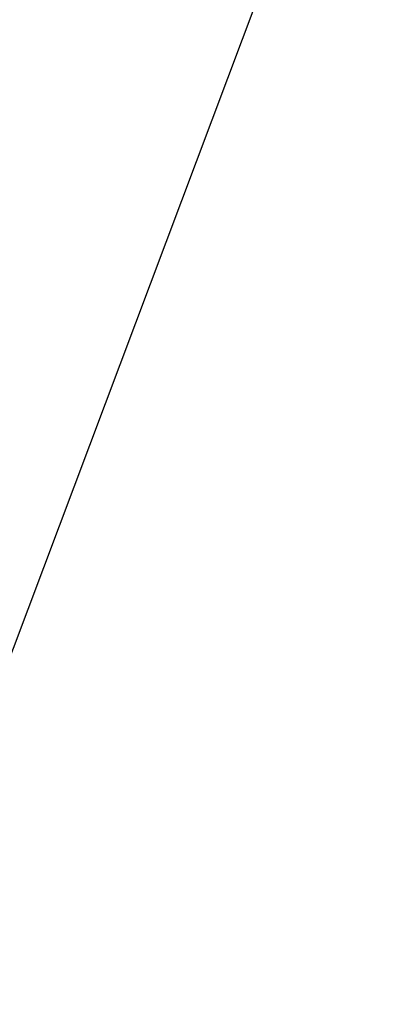
# Model space of a CAD drawing. Units: inches. Extents: x 3590 to 5167, y 65 to 1917.
# Tile 86 of 100: x 5051.6658 to 5051.8188, y 1788.6144 to 1789.0318. Entities that reach past the tile are written whole.
import ezdxf

# ---------------------------------------------------------------- set-up
doc = ezdxf.new("R2010")
doc.units = ezdxf.units.IN
for name, color, linetype, lineweight in [('A-ANNO-DIMS', 2, 'Continuous', 18), ('A-FLOR-PATT', 8, 'Continuous', 13), ('L-PLNT', 94, 'Continuous', 18)]:
    doc.layers.add(name, color=color, linetype=linetype, lineweight=lineweight)
doc.layers.add('DIENHOA', color=3, linetype='Continuous')
doc.styles.get("Standard").update_dxf_attribs({"font": 'arial.ttf'})
doc.dimstyles.new('ISO-25', dxfattribs={"dimtxt": 9, "dimasz": 2.5, "dimexe": 1.25, "dimexo": 0.625, "dimtad": 1, "dimdec": 1, "dimlunit": 3, "dimtxsty": 'Standard', "dimcen": 2.5, "dimadec": 0, "dimazin": 0, "dimtfac": 1, "dimtdec": 1, "dimtmove": 0, "dimatfit": 3, "dimfxl": 1, "dimarcsym": 0})

# ---------------------------------------------------------------- blocks, each defined once
blk = doc.blocks.new('Cay03_mb')
at = {"layer": 'DIENHOA'}
blk.add_lwpolyline([(23.687, -5.439), (19.839, 92.987), (20.283, 176.968), (25.016, 248.547), (34.033, 309.769), (47.331, 362.677), (64.906, 409.313), (86.753, 451.722), (112.868, 491.948)], dxfattribs=at)
blk = doc.blocks.new('*D323')
at = {"layer": 'A-ANNO-DIMS', "color": 0, "lineweight": -2, "transparency": 16777216}
for p, q in [((5069.17227, 1795.21603), (5069.17227, 1874.95034)), ((5065.43703, 1795.21603), (5070.42227, 1795.21603)), ((5069.17227, 1769.30924), (5069.17227, 1792.71603)), ((5065.43703, 1766.80924), (5070.42227, 1766.80924))]:
    blk.add_line(p, q, dxfattribs=at)
at = {"layer": 'A-ANNO-DIMS', "color": 0, "transparency": 16777216}
for points in [[(5068.75561, 1792.71603), (5069.58894, 1792.71603), (5069.17227, 1795.21603)], [(5068.75561, 1769.30924), (5069.58894, 1769.30924), (5069.17227, 1766.80924)]]:
    blk.add_solid(points, dxfattribs=at)
at = {"layer": 'Defpoints', "color": 0, "transparency": 16777216}
for p in [(5064.81203, 1795.21603), (5069.17227, 1795.21603), (5064.81203, 1766.80924)]:
    blk.add_point(p, dxfattribs=at)
at = {"layer": 'A-ANNO-DIMS', "color": 0, "transparency": 16777216, "insert": (5063.89379, 1836.33318), "char_height": 9, "attachment_point": 5, "rotation": 90}
blk.add_mtext('2\'-4 1/2" TYP.', dxfattribs=at)

msp = doc.modelspace()

# ---------------------------------------------------------------- hatches: boundary and pattern name
at = {"layer": 'A-FLOR-PATT', "transparency": 33554687}
h = msp.add_hatch(dxfattribs=at)
h.set_pattern_fill('AR-HBONE', color=256, scale=0.2)
h.set_pattern_definition([(45, (-588.972, 0), (0, 28.73682), [60.96, -20.32]), (135, (-574.604, 14.368), (3e-15, 28.73682), [60.96, -20.32])])
h.paths.add_polyline_path([(5071.27403, 1796.99898), (4933.27403, 1796.99898), (4933.27403, 1753.99898), (4962.77403, 1753.99898, -0.414214), (4928.77403, 1719.99898), (4933.27403, 1718.99898), (4933.27403, 1334.99898), (5071.27403, 1334.99898)])
h.paths.add_polyline_path([(4951.78002, 1521.0767), (4951.7151, 1521.0404), (4951.56345, 1520.89532)], flags=16)
h.paths.add_polyline_path([(4952.267, 1521.37645), (4952.1977, 1521.37111), (4952.19823, 1521.35558)], flags=0)
h.paths.add_polyline_path([(4967.05076, 1529.72832), (4965.23122, 1528.69444), (4963.41109, 1527.71401), (4961.75649, 1526.85081), (4963.58887, 1527.44938), (4964.03555, 1527.47802), (4962.9755, 1527.24902), (4961.76022, 1526.85203), (4959.79219, 1525.83406), (4958.00498, 1524.89483), (4956.24031, 1523.92961), (4954.50395, 1522.91854), (4954.1294, 1522.68163), (4953.36051, 1521.99688), (4953.36558, 1521.99754), (4953.605, 1522.06367), (4955.10605, 1522.76083), (4956.92108, 1523.43405), (4958.67784, 1523.91513), (4960.35834, 1524.20036), (4961.94456, 1524.28606), (4964.17144, 1524.10849), (4965.95752, 1523.30903), (4963.86273, 1522.97565), (4965.18742, 1522.49898), (4963.36614, 1522.49715), (4961.54526, 1522.48682), (4959.76359, 1522.46077), (4958.30414, 1522.4188), (4957.97356, 1522.38829), (4956.30692, 1522.2324), (4954.71821, 1522.07143), (4953.25077, 1521.89915), (4953.52509, 1521.62277), (4954.33087, 1521.37883), (4956.24263, 1521.22987), (4958.03913, 1520.92952), (4959.68424, 1520.48339), (4961.16007, 1519.89569), (4963.10699, 1518.80022), (4964.39286, 1517.32518), (4962.97306, 1517.72596), (4964.55841, 1516.66059), (4965.40664, 1515.70779), (4963.50733, 1516.32179), (4961.67995, 1517.0051), (4959.93478, 1517.74489), (4958.2821, 1518.52833), (4956.73216, 1519.34257), (4955.29527, 1520.17478), (4954.67155, 1520.57237), (4954.51279, 1520.6271), (4955.65848, 1519.31837), (4956.70263, 1517.98232), (4957.64403, 1516.64663), (4958.48545, 1515.33439), (4959.54998, 1513.52398), (4960.43768, 1511.76936), (4958.84107, 1513.6196), (4957.45175, 1515.3249), (4955.8186, 1517.45855), (4956.66537, 1515.44764), (4957.11109, 1513.92292), (4957.44681, 1511.71434), (4957.07641, 1509.79288), (4956.53757, 1511.1103), (4955.99231, 1512.56892), (4955.44448, 1514.12509), (4954.89794, 1515.73518), (4954.35653, 1517.35553), (4953.82412, 1518.94251), (4953.30455, 1520.45247), (4953.06452, 1521.11563), (4952.97143, 1521.14607), (4952.94932, 1521.08646), (4952.72981, 1520.19905), (4953.3698, 1518.02364), (4953.75708, 1516.37279), (4954.05124, 1514.76538), (4954.26449, 1513.22121), (4954.47124, 1511.13121), (4954.4971, 1510.40174), (4954.40903, 1511.76006), (4954.26449, 1513.22121), (4954.05124, 1514.76538), (4953.75708, 1516.37279), (4953.3698, 1518.02364), (4952.87718, 1519.69813), (4952.7161, 1520.1412), (4952.53301, 1519.05871), (4952.37428, 1517.78881), (4952.21925, 1516.31167), (4952.04598, 1514.59986), (4951.83253, 1512.62598), (4951.55697, 1510.36259), (4951.20331, 1512.16818), (4950.85168, 1514.33931), (4950.98529, 1516.37594), (4951.6596, 1518.28625), (4952.59261, 1520.48085), (4952.35664, 1521.1299), (4951.85502, 1520.32753), (4950.83901, 1518.90828), (4949.77675, 1517.58658), (4948.91554, 1516.61731), (4948.11099, 1515.2561), (4947.0891, 1513.55389), (4945.88937, 1511.61495), (4946.32587, 1513.40232), (4946.5624, 1514.24913), (4945.52771, 1513.32668), (4944.58105, 1512.53126), (4946.01774, 1514.50825), (4947.2044, 1516.04763), (4947.89331, 1517.31331), (4949.30686, 1518.76446), (4950.41417, 1519.76716), (4950.45131, 1519.80628), (4952.267, 1521.37645), (4951.64457, 1521.49317), (4950.40371, 1521.17954), (4948.04447, 1520.35868), (4946.11863, 1519.45198), (4944.57182, 1518.47484), (4943.34962, 1517.44265), (4941.99695, 1515.91971), (4941.66146, 1515.27475), (4942.81332, 1516.98973), (4944.57182, 1518.47484), (4946.11863, 1519.45198), (4948.04447, 1520.35868), (4950.40371, 1521.17954), (4951.64457, 1521.49317), (4949.64678, 1521.86781), (4948.59979, 1521.75633), (4947.12629, 1521.5699), (4945.42015, 1521.34763), (4943.44969, 1521.10462), (4941.18319, 1520.85596), (4942.86028, 1521.61265), (4943.87308, 1522.03014), (4942.95216, 1521.9093), (4941.40968, 1521.48512), (4939.54287, 1520.67019), (4938.96775, 1520.2255), (4940.73284, 1521.29899), (4942.95216, 1521.9093), (4943.70184, 1522.00767), (4945.89419, 1522.69998), (4947.56488, 1522.71399), (4948.92086, 1522.56573), (4951.13144, 1522.18271), (4950.97062, 1522.2969), (4948.12924, 1523.00563), (4946.03496, 1523.70671), (4944.23235, 1524.52143), (4942.70692, 1525.46111), (4941.44419, 1526.53707), (4940.42968, 1527.76062), (4939.6489, 1529.14306), (4941.42091, 1528.12232), (4943.14742, 1527.13248), (4944.84093, 1526.17457), (4946.51394, 1525.24959), (4948.17893, 1524.35855), (4948.36457, 1524.26336), (4946.47531, 1526.04459), (4945.18083, 1527.54042), (4944.19039, 1529.03339), (4943.49559, 1530.53985), (4943.27808, 1531.3597), (4942.49849, 1531.91903), (4943.11353, 1531.76249), (4942.95927, 1533.6586), (4944.13953, 1531.9886), (4944.61171, 1531.32339), (4946.20163, 1530.46341), (4947.48567, 1529.50925), (4948.79027, 1528.22649), (4950.36754, 1526.23746), (4949.48547, 1528.15549), (4948.85128, 1530.12254), (4948.49054, 1532.04127), (4948.38105, 1533.91822), (4948.50062, 1535.7599), (4948.82704, 1537.57284), (4949.41803, 1535.56526), (4949.95684, 1533.56932), (4950.46414, 1531.5861), (4950.96058, 1529.6167), (4951.3911, 1527.95448), (4951.72352, 1530.68689), (4952.20106, 1532.57994), (4952.88914, 1534.32964), (4953.77035, 1535.95123), (4954.82726, 1537.45995), (4954.52145, 1535.38966), (4954.27314, 1533.93684), (4955.57999, 1535.6627), (4956.74758, 1536.73859), (4956.15852, 1534.78029), (4955.58917, 1532.87334), (4955.04336, 1531.00581), (4954.52493, 1529.16576), (4954.03771, 1527.34127), (4953.63833, 1525.73298), (4953.61143, 1525.58564), (4953.39805, 1524.16565), (4953.38219, 1524.00887), (4954.06955, 1525.47563), (4954.91212, 1527.02173), (4956.13627, 1528.89351), (4957.84668, 1530.57701), (4959.37601, 1531.54014), (4958.25596, 1530.10398), (4957.14284, 1528.66291), (4956.06626, 1527.24305), (4955.05579, 1525.87054), (4954.14104, 1524.57149), (4953.35159, 1523.37204), (4953.31079, 1523.30299), (4953.27253, 1522.92478), (4953.26102, 1522.38213), (4954.1031, 1523.37273), (4954.63005, 1524.28376), (4955.96149, 1526.35767), (4957.23002, 1528.12969), (4958.42057, 1529.60864), (4960.03671, 1531.36792), (4961.3736, 1532.3752), (4962.1015, 1532.77), (4961.06994, 1531.06113), (4959.98733, 1529.43811), (4958.86851, 1527.90803), (4958.15046, 1527.00742), (4959.80291, 1528.00314), (4961.58854, 1528.79257), (4963.39087, 1529.32783), (4965.21118, 1529.63205)], flags=16)
h.paths.add_polyline_path([(4962.94387, 1523.18187), (4961.10714, 1523.42192), (4960.39205, 1523.36158), (4962.34964, 1523.33061)], flags=0)
h.paths.add_polyline_path([(5049.54129, 1584.55089), (5049.47636, 1584.51458), (5049.32471, 1584.3695)], flags=16)
h.paths.add_polyline_path([(5050.02827, 1584.85063), (5049.95897, 1584.84529), (5049.95949, 1584.82976)], flags=0)
h.paths.add_polyline_path([(5042.33308, 1581.94902), (5043.8799, 1582.92616), (5045.80573, 1583.83286), (5048.16498, 1584.65372), (5049.40583, 1584.96736), (5047.40804, 1585.34199), (5046.36106, 1585.23052), (5044.88755, 1585.04408), (5043.18142, 1584.82181), (5041.21095, 1584.5788), (5038.94446, 1584.33014), (5040.62155, 1585.08683), (5041.63434, 1585.50432), (5040.71343, 1585.38348), (5039.17095, 1584.9593), (5037.30414, 1584.14438), (5036.72901, 1583.69969), (5038.4941, 1584.77317), (5040.71343, 1585.38348), (5041.4631, 1585.48185), (5043.65545, 1586.17416), (5045.32615, 1586.18818), (5046.68212, 1586.03992), (5048.8927, 1585.6569), (5048.73188, 1585.77108), (5045.89051, 1586.47981), (5043.79622, 1587.18089), (5041.99361, 1587.99561), (5040.46818, 1588.9353), (5039.20546, 1590.01125), (5038.19095, 1591.2348), (5037.41016, 1592.61725), (5039.18217, 1591.5965), (5040.90868, 1590.60667), (5042.6022, 1589.64876), (5044.2752, 1588.72378), (5045.94019, 1587.83274), (5046.12584, 1587.73754), (5044.23658, 1589.51878), (5042.9421, 1591.01461), (5041.95166, 1592.50757), (5041.25685, 1594.01403), (5041.03935, 1594.83388), (5040.25976, 1595.39321), (5040.8748, 1595.23667), (5040.72054, 1597.13279), (5041.9008, 1595.46278), (5042.37297, 1594.79758), (5043.96289, 1593.93759), (5045.24694, 1592.98344), (5046.55153, 1591.70068), (5048.12881, 1589.71164), (5047.24673, 1591.62967), (5046.61254, 1593.59672), (5046.2518, 1595.51546), (5046.14232, 1597.3924), (5046.26189, 1599.23408), (5046.5883, 1601.04703), (5047.17929, 1599.03944), (5047.71811, 1597.0435), (5048.22541, 1595.06028), (5048.72184, 1593.09089), (5049.15237, 1591.42866), (5049.48478, 1594.16107), (5049.96233, 1596.05412), (5050.65041, 1597.80382), (5051.53161, 1599.42541), (5052.58852, 1600.93414), (5052.28271, 1598.86384), (5052.03441, 1597.41102), (5053.34126, 1599.13689), (5054.50884, 1600.21277), (5053.91979, 1598.25447), (5053.35044, 1596.34752), (5052.80463, 1594.47999), (5052.2862, 1592.63995), (5051.79898, 1590.81546), (5051.39959, 1589.20716), (5051.3727, 1589.05983), (5051.15931, 1587.63984), (5051.14346, 1587.48305), (5051.83082, 1588.94982), (5052.67339, 1590.49592), (5053.89754, 1592.3677), (5055.60794, 1594.05119), (5057.13728, 1595.01432), (5056.01722, 1593.57817), (5054.90411, 1592.1371), (5053.82752, 1590.71724), (5052.81705, 1589.34472), (5051.9023, 1588.04567), (5051.11286, 1586.84622), (5051.07205, 1586.77718), (5051.03379, 1586.39896), (5051.02228, 1585.85631), (5051.86437, 1586.84692), (5052.39131, 1587.75794), (5053.72275, 1589.83185), (5054.99128, 1591.60387), (5056.18183, 1593.08282), (5057.79798, 1594.84211), (5059.13486, 1595.84938), (5059.86276, 1596.24419), (5058.83121, 1594.53531), (5057.7486, 1592.9123), (5056.62978, 1591.38221), (5055.91173, 1590.4816), (5057.56418, 1591.47732), (5059.34981, 1592.26675), (5061.15214, 1592.80202), (5062.97245, 1593.10624), (5064.81203, 1593.20251), (5062.99248, 1592.16863), (5061.17235, 1591.18819), (5059.51775, 1590.325), (5061.35014, 1590.92356), (5061.79682, 1590.95221), (5060.73676, 1590.7232), (5059.52148, 1590.32622), (5057.55345, 1589.30825), (5055.76625, 1588.36901), (5054.00157, 1587.40379), (5052.26521, 1586.39273), (5051.89067, 1586.15581), (5051.12177, 1585.47106), (5051.12684, 1585.47172), (5051.36627, 1585.53786), (5052.86732, 1586.23502), (5054.68234, 1586.90824), (5056.4391, 1587.38931), (5058.1196, 1587.67454), (5059.70582, 1587.76024), (5061.93271, 1587.58268), (5063.71878, 1586.78321), (5061.62399, 1586.44983), (5062.94869, 1585.97317), (5061.12741, 1585.97133), (5059.30653, 1585.961), (5057.52486, 1585.93496), (5056.06541, 1585.89299), (5055.73482, 1585.86247), (5054.06819, 1585.70658), (5052.47947, 1585.54561), (5051.01204, 1585.37333), (5051.28635, 1585.09695), (5052.09214, 1584.85301), (5054.00389, 1584.70406), (5055.8004, 1584.4037), (5057.44551, 1583.95757), (5058.92133, 1583.36987), (5060.86825, 1582.27441), (5062.15413, 1580.79937), (5060.73433, 1581.20015), (5062.31967, 1580.13477), (5063.1679, 1579.18198), (5061.2686, 1579.79597), (5059.44122, 1580.47928), (5057.69605, 1581.21908), (5056.04336, 1582.00251), (5054.49343, 1582.81675), (5053.05653, 1583.64897), (5052.43281, 1584.04656), (5052.27405, 1584.10128), (5053.41974, 1582.79255), (5054.4639, 1581.4565), (5055.40529, 1580.12081), (5056.24672, 1578.80858), (5057.31125, 1576.99816), (5058.19895, 1575.24354), (5056.60234, 1577.09378), (5055.21301, 1578.79908), (5053.57987, 1580.93274), (5054.42664, 1578.92183), (5054.87235, 1577.3971), (5055.20808, 1575.18852), (5054.83767, 1573.26706), (5054.29883, 1574.58448), (5053.75357, 1576.0431), (5053.20575, 1577.59927), (5052.6592, 1579.20936), (5052.1178, 1580.82971), (5051.58538, 1582.41669), (5051.06582, 1583.92666), (5050.82578, 1584.58981), (5050.7327, 1584.62025), (5050.71058, 1584.56064), (5050.49108, 1583.67323), (5051.13107, 1581.49782), (5051.51835, 1579.84698), (5051.8125, 1578.23957), (5052.02575, 1576.69539), (5052.23251, 1574.6054), (5052.25836, 1573.87593), (5052.1703, 1575.23424), (5052.02575, 1576.69539), (5051.8125, 1578.23957), (5051.51835, 1579.84698), (5051.13107, 1581.49782), (5050.63844, 1583.17231), (5050.47736, 1583.61538), (5050.29428, 1582.53289), (5050.13554, 1581.26299), (5049.98051, 1579.78585), (5049.80724, 1578.07405), (5049.59379, 1576.10016), (5049.31823, 1573.83678), (5048.96458, 1575.64237), (5048.61294, 1577.8135), (5048.74656, 1579.85012), (5049.42086, 1581.76043), (5050.35388, 1583.95503), (5050.1179, 1584.60408), (5049.61629, 1583.80172), (5048.60027, 1582.38246), (5047.53801, 1581.06076), (5046.67681, 1580.09149), (5045.87225, 1578.73029), (5044.85036, 1577.02808), (5043.65063, 1575.08913), (5044.08713, 1576.8765), (5044.32366, 1577.72331), (5043.28898, 1576.80086), (5042.34232, 1576.00545), (5043.779, 1577.98243), (5044.96566, 1579.52182), (5045.65457, 1580.78749), (5047.06813, 1582.23865), (5048.17543, 1583.24134), (5048.21258, 1583.28047), (5050.02827, 1584.85063), (5049.40583, 1584.96736), (5048.16498, 1584.65372), (5045.80573, 1583.83286), (5043.8799, 1582.92616), (5042.33308, 1581.94902), (5041.11088, 1580.91684), (5039.75821, 1579.39389), (5039.42272, 1578.74894), (5040.57458, 1580.46391)], flags=16)
h.paths.add_polyline_path([(4954.79872, 1533.12029), (4954.26249, 1532.07935), (4953.83112, 1530.93464), (4953.50472, 1529.63602), (4953.28338, 1528.13331), (4953.16721, 1526.37637), (4953.15631, 1524.31504), (4953.27669, 1521.23629), (4952.80168, 1521.84177), (4951.55695, 1521.99789), (4950.97575, 1521.9613), (4952.66059, 1521.94097), (4952.80168, 1521.84177), (4953.15249, 1523.59258), (4953.16721, 1526.37637), (4953.28338, 1528.13331), (4953.60929, 1530.34598), (4954.45558, 1532.59174)], flags=0)
h.paths.add_polyline_path([(5050.56294, 1585.31596), (5049.31822, 1585.47208), (5048.73702, 1585.43548), (5050.42186, 1585.41516), (5050.56294, 1585.31596), (5050.91375, 1587.06676), (5050.92848, 1589.85056), (5051.04465, 1591.6075), (5051.37055, 1593.82017), (5052.21684, 1596.06593), (5052.55999, 1596.59447), (5052.02375, 1595.55353), (5051.59238, 1594.40883), (5051.26598, 1593.1102), (5051.04465, 1591.6075), (5050.92848, 1589.85056), (5050.91757, 1587.78922), (5051.03795, 1584.71048)], flags=0)
h.paths.add_polyline_path([(5058.15332, 1586.83576), (5060.11091, 1586.80479), (5060.70514, 1586.65605), (5058.8684, 1586.8961)], flags=0)
h.paths.add_polyline_path([(5049.54129, 1430.93611), (5049.47636, 1430.8998), (5049.32471, 1430.75472)], flags=16)
h.paths.add_polyline_path([(5050.02827, 1431.23585), (5049.95897, 1431.23051), (5049.95949, 1431.21498)], flags=0)
h.paths.add_polyline_path([(5046.5883, 1447.43225), (5047.17929, 1445.42467), (5047.71811, 1443.42872), (5048.22541, 1441.4455), (5048.72184, 1439.47611), (5049.15237, 1437.81388), (5049.48478, 1440.5463), (5049.96233, 1442.43934), (5050.65041, 1444.18904), (5051.53161, 1445.81063), (5052.58852, 1447.31936), (5052.28271, 1445.24906), (5052.03441, 1443.79624), (5053.34126, 1445.52211), (5054.50884, 1446.59799), (5053.91979, 1444.63969), (5053.35044, 1442.73274), (5052.80463, 1440.86521), (5052.2862, 1439.02517), (5051.79898, 1437.20068), (5051.39959, 1435.59238), (5051.3727, 1435.44505), (5051.15931, 1434.02506), (5051.14346, 1433.86828), (5051.83082, 1435.33504), (5052.67339, 1436.88114), (5053.89754, 1438.75292), (5055.60794, 1440.43641), (5057.13728, 1441.39954), (5056.01722, 1439.96339), (5054.90411, 1438.52232), (5053.82752, 1437.10246), (5052.81705, 1435.72994), (5051.9023, 1434.4309), (5051.11286, 1433.23145), (5051.07205, 1433.1624), (5051.03379, 1432.78418), (5051.02228, 1432.24153), (5051.86437, 1433.23214), (5052.39131, 1434.14316), (5053.72275, 1436.21707), (5054.99128, 1437.98909), (5056.18183, 1439.46805), (5057.79798, 1441.22733), (5059.13486, 1442.23461), (5059.86276, 1442.62941), (5058.83121, 1440.92053), (5057.7486, 1439.29752), (5056.62978, 1437.76743), (5055.91173, 1436.86682), (5057.56418, 1437.86255), (5059.34981, 1438.65197), (5061.15214, 1439.18724), (5062.97245, 1439.49146), (5064.81203, 1439.58773), (5062.99248, 1438.55385), (5061.17235, 1437.57342), (5059.51775, 1436.71022), (5061.35014, 1437.30879), (5061.79682, 1437.33743), (5060.73676, 1437.10842), (5059.52148, 1436.71144), (5057.55345, 1435.69347), (5055.76625, 1434.75423), (5054.00157, 1433.78901), (5052.26521, 1432.77795), (5051.89067, 1432.54103), (5051.12177, 1431.85628), (5051.12684, 1431.85694), (5051.36627, 1431.92308), (5052.86732, 1432.62024), (5054.68234, 1433.29346), (5056.4391, 1433.77453), (5058.1196, 1434.05976), (5059.70582, 1434.14546), (5061.93271, 1433.9679), (5063.71878, 1433.16843), (5061.62399, 1432.83505), (5062.94869, 1432.35839), (5061.12741, 1432.35655), (5059.30653, 1432.34623), (5057.52486, 1432.32018), (5056.06541, 1432.27821), (5055.73482, 1432.24769), (5054.06819, 1432.09181), (5052.47947, 1431.93083), (5051.01204, 1431.75856), (5051.28635, 1431.48218), (5052.09214, 1431.23823), (5054.00389, 1431.08928), (5055.8004, 1430.78892), (5057.44551, 1430.34279), (5058.92133, 1429.75509), (5060.86825, 1428.65963), (5062.15413, 1427.18459), (5060.73433, 1427.58537), (5062.31967, 1426.52), (5063.1679, 1425.5672), (5061.2686, 1426.18119), (5059.44122, 1426.86451), (5057.69605, 1427.6043), (5056.04336, 1428.38773), (5054.49343, 1429.20197), (5053.05653, 1430.03419), (5052.43281, 1430.43178), (5052.27405, 1430.48651), (5053.41974, 1429.17777), (5054.4639, 1427.84172), (5055.40529, 1426.50603), (5056.24672, 1425.1938), (5057.31125, 1423.38338), (5058.19895, 1421.62877), (5056.60234, 1423.479), (5055.21301, 1425.1843), (5053.57987, 1427.31796), (5054.42664, 1425.30705), (5054.87235, 1423.78233), (5055.20808, 1421.57374), (5054.83767, 1419.65228), (5054.29883, 1420.9697), (5053.75357, 1422.42832), (5053.20575, 1423.9845), (5052.6592, 1425.59458), (5052.1178, 1427.21493), (5051.58538, 1428.80191), (5051.06582, 1430.31188), (5050.82578, 1430.97503), (5050.7327, 1431.00547), (5050.71058, 1430.94586), (5050.49108, 1430.05845), (5051.13107, 1427.88305), (5051.51835, 1426.2322), (5051.8125, 1424.62479), (5052.02575, 1423.08061), (5052.23251, 1420.99062), (5052.25836, 1420.26115), (5052.1703, 1421.61947), (5052.02575, 1423.08061), (5051.8125, 1424.62479), (5051.51835, 1426.2322), (5051.13107, 1427.88305), (5050.63844, 1429.55753), (5050.47736, 1430.0006), (5050.29428, 1428.91811), (5050.13554, 1427.64821), (5049.98051, 1426.17107), (5049.80724, 1424.45927), (5049.59379, 1422.48539), (5049.31823, 1420.222), (5048.96458, 1422.02759), (5048.61294, 1424.19872), (5048.74656, 1426.23534), (5049.42086, 1428.14565), (5050.35388, 1430.34025), (5050.1179, 1430.98931), (5049.61629, 1430.18694), (5048.60027, 1428.76768), (5047.53801, 1427.44598), (5046.67681, 1426.47671), (5045.87225, 1425.11551), (5044.85036, 1423.4133), (5043.65063, 1421.47435), (5044.08713, 1423.26172), (5044.32366, 1424.10854), (5043.28898, 1423.18608), (5042.34232, 1422.39067), (5043.779, 1424.36765), (5044.96566, 1425.90704), (5045.65457, 1427.17272), (5047.06813, 1428.62387), (5048.17543, 1429.62657), (5048.21258, 1429.66569), (5050.02827, 1431.23585), (5049.40583, 1431.35258), (5048.16498, 1431.03894), (5045.80573, 1430.21809), (5043.8799, 1429.31139), (5042.33308, 1428.33424), (5041.11088, 1427.30206), (5039.75821, 1425.77911), (5039.42272, 1425.13416), (5040.57458, 1426.84914), (5042.33308, 1428.33424), (5043.8799, 1429.31139), (5045.80573, 1430.21809), (5048.16498, 1431.03894), (5049.40583, 1431.35258), (5047.40804, 1431.72722), (5046.36106, 1431.61574), (5044.88755, 1431.42931), (5043.18142, 1431.20704), (5041.21095, 1430.96402), (5038.94446, 1430.71536), (5040.62155, 1431.47205), (5041.63434, 1431.88954), (5040.71343, 1431.76871), (5039.17095, 1431.34453), (5037.30414, 1430.5296), (5036.72901, 1430.08491), (5038.4941, 1431.1584), (5040.71343, 1431.76871), (5041.4631, 1431.86707), (5043.65545, 1432.55939), (5045.32615, 1432.5734), (5046.68212, 1432.42514), (5048.8927, 1432.04212), (5048.73188, 1432.1563), (5045.89051, 1432.86503), (5043.79622, 1433.56611), (5041.99361, 1434.38083), (5040.46818, 1435.32052), (5039.20546, 1436.39648), (5038.19095, 1437.62002), (5037.41016, 1439.00247), (5039.18217, 1437.98172), (5040.90868, 1436.99189), (5042.6022, 1436.03398), (5044.2752, 1435.109), (5045.94019, 1434.21796), (5046.12584, 1434.12276), (5044.23658, 1435.904), (5042.9421, 1437.39983), (5041.95166, 1438.8928), (5041.25685, 1440.39925), (5041.03935, 1441.2191), (5040.25976, 1441.77844), (5040.8748, 1441.62189), (5040.72054, 1443.51801), (5041.9008, 1441.848), (5042.37297, 1441.1828), (5043.96289, 1440.32282), (5045.24694, 1439.36866), (5046.55153, 1438.0859), (5048.12881, 1436.09686), (5047.24673, 1438.01489), (5046.61254, 1439.98195), (5046.2518, 1441.90068), (5046.14232, 1443.77762), (5046.26189, 1445.6193)], flags=16)
h.paths.add_polyline_path([(5052.38176, 1444.25496), (5051.62263, 1442.77987), (5052.02375, 1441.93875), (5052.55999, 1442.9797)], flags=0)
h.paths.add_polyline_path([(5050.56294, 1431.70118), (5049.31822, 1431.8573), (5048.73702, 1431.82071), (5050.42186, 1431.80038)], flags=0)
h.paths.add_polyline_path([(5058.15332, 1433.22098), (5060.11091, 1433.19001), (5060.70514, 1433.04127), (5058.8684, 1433.28132)], flags=0)
h.paths.add_polyline_path([(5049.54129, 1352.28535), (5049.47636, 1352.24904), (5049.32471, 1352.10396)], flags=16)
h.paths.add_polyline_path([(5050.02827, 1352.58509), (5049.95897, 1352.57975), (5049.95949, 1352.56422)], flags=0)
h.paths.add_polyline_path([(5046.5883, 1368.78149), (5047.17929, 1366.7739), (5047.71811, 1364.77796), (5048.22541, 1362.79474), (5048.72184, 1360.82534), (5049.15237, 1359.16312), (5049.48478, 1361.89553), (5049.96233, 1363.78858), (5050.65041, 1365.53828), (5051.53161, 1367.15987), (5052.58852, 1368.6686), (5052.28271, 1366.5983), (5052.03441, 1365.14548), (5053.34126, 1366.87135), (5054.50884, 1367.94723), (5053.91979, 1365.98893), (5053.35044, 1364.08198), (5052.80463, 1362.21445), (5052.2862, 1360.37441), (5051.79898, 1358.54992), (5051.39959, 1356.94162), (5051.3727, 1356.79428), (5051.15931, 1355.37429), (5051.14346, 1355.21751), (5051.83082, 1356.68428), (5052.67339, 1358.23037), (5053.89754, 1360.10216), (5055.60794, 1361.78565), (5057.13728, 1362.74878), (5056.01722, 1361.31262), (5054.90411, 1359.87155), (5053.82752, 1358.4517), (5052.81705, 1357.07918), (5051.9023, 1355.78013), (5051.11286, 1354.58068), (5051.07205, 1354.51164), (5051.03379, 1354.13342), (5051.02228, 1353.59077), (5051.86437, 1354.58137), (5052.39131, 1355.4924), (5053.72275, 1357.56631), (5054.99128, 1359.33833), (5056.18183, 1360.81728), (5057.79798, 1362.57656), (5059.13486, 1363.58384), (5059.86276, 1363.97864), (5058.83121, 1362.26977), (5057.7486, 1360.64675), (5056.62978, 1359.11667), (5055.91173, 1358.21606), (5057.56418, 1359.21178), (5059.34981, 1360.00121), (5061.15214, 1360.53648), (5062.97245, 1360.84069), (5064.81203, 1360.93697), (5062.99248, 1359.90308), (5061.17235, 1358.92265), (5059.51775, 1358.05946), (5061.35014, 1358.65802), (5061.79682, 1358.68666), (5060.73676, 1358.45766), (5059.52148, 1358.06068), (5057.55345, 1357.0427), (5055.76625, 1356.10347), (5054.00157, 1355.13825), (5052.26521, 1354.12718), (5051.89067, 1353.89027), (5051.12177, 1353.20552), (5051.12684, 1353.20618), (5051.36627, 1353.27231), (5052.86732, 1353.96947), (5054.68234, 1354.6427), (5056.4391, 1355.12377), (5058.1196, 1355.409), (5059.70582, 1355.4947), (5061.93271, 1355.31713), (5063.71878, 1354.51767), (5061.62399, 1354.18429), (5062.94869, 1353.70763), (5061.12741, 1353.70579), (5059.30653, 1353.69546), (5057.52486, 1353.66942), (5056.06541, 1353.62744), (5055.73482, 1353.59693), (5054.06819, 1353.44104), (5052.47947, 1353.28007), (5051.01204, 1353.10779), (5051.28635, 1352.83141), (5052.09214, 1352.58747), (5054.00389, 1352.43852), (5055.8004, 1352.13816), (5057.44551, 1351.69203), (5058.92133, 1351.10433), (5060.86825, 1350.00887), (5062.15413, 1348.53382), (5060.73433, 1348.9346), (5062.31967, 1347.86923), (5063.1679, 1346.91643), (5061.2686, 1347.53043), (5059.44122, 1348.21374), (5057.69605, 1348.95353), (5056.04336, 1349.73697), (5054.49343, 1350.55121), (5053.05653, 1351.38342), (5052.43281, 1351.78101), (5052.27405, 1351.83574), (5053.41974, 1350.52701), (5054.4639, 1349.19096), (5055.40529, 1347.85527), (5056.24672, 1346.54303), (5057.31125, 1344.73262), (5058.19895, 1342.978), (5056.60234, 1344.82824), (5055.21301, 1346.53354), (5053.57987, 1348.6672), (5054.42664, 1346.65629), (5054.87235, 1345.13156), (5055.20808, 1342.92298), (5054.83767, 1341.00152), (5054.29883, 1342.31894), (5053.75357, 1343.77756), (5053.20575, 1345.33373), (5052.6592, 1346.94382), (5052.1178, 1348.56417), (5051.58538, 1350.15115), (5051.06582, 1351.66111), (5050.82578, 1352.32427), (5050.7327, 1352.35471), (5050.71058, 1352.2951), (5050.49108, 1351.40769), (5051.13107, 1349.23228), (5051.51835, 1347.58144), (5051.8125, 1345.97403), (5052.02575, 1344.42985), (5052.23251, 1342.33986), (5052.25836, 1341.61039), (5052.1703, 1342.9687), (5052.02575, 1344.42985), (5051.8125, 1345.97403), (5051.51835, 1347.58144), (5051.13107, 1349.23228), (5050.63844, 1350.90677), (5050.47736, 1351.34984), (5050.29428, 1350.26735), (5050.13554, 1348.99745), (5049.98051, 1347.52031), (5049.80724, 1345.80851), (5049.59379, 1343.83462), (5049.31823, 1341.57124), (5048.96458, 1343.37683), (5048.61294, 1345.54796), (5048.74656, 1347.58458), (5049.42086, 1349.49489), (5050.35388, 1351.68949), (5050.1179, 1352.33854), (5049.61629, 1351.53617), (5048.60027, 1350.11692), (5047.53801, 1348.79522), (5046.67681, 1347.82595), (5045.87225, 1346.46475), (5044.85036, 1344.76253), (5043.65063, 1342.82359), (5044.08713, 1344.61096), (5044.32366, 1345.45777), (5043.28898, 1344.53532), (5042.34232, 1343.7399), (5043.779, 1345.71689), (5044.96566, 1347.25627), (5045.65457, 1348.52195), (5047.06813, 1349.9731), (5048.17543, 1350.9758), (5048.21258, 1351.01493), (5050.02827, 1352.58509), (5049.40583, 1352.70181), (5048.16498, 1352.38818), (5045.80573, 1351.56732), (5043.8799, 1350.66062), (5042.33308, 1349.68348), (5041.11088, 1348.65129), (5039.75821, 1347.12835), (5039.42272, 1346.4834), (5040.57458, 1348.19837), (5042.33308, 1349.68348), (5043.8799, 1350.66062), (5045.80573, 1351.56732), (5048.16498, 1352.38818), (5049.40583, 1352.70181), (5047.40804, 1353.07645), (5046.36106, 1352.96498), (5044.88755, 1352.77854), (5043.18142, 1352.55627), (5041.21095, 1352.31326), (5038.94446, 1352.0646), (5040.62155, 1352.82129), (5041.63434, 1353.23878), (5040.71343, 1353.11794), (5039.17095, 1352.69376), (5037.30414, 1351.87884), (5036.72901, 1351.43415), (5038.4941, 1352.50763), (5040.71343, 1353.11794), (5041.4631, 1353.21631), (5043.65545, 1353.90862), (5045.32615, 1353.92263), (5046.68212, 1353.77438), (5048.8927, 1353.39136), (5048.73188, 1353.50554), (5045.89051, 1354.21427), (5043.79622, 1354.91535), (5041.99361, 1355.73007), (5040.46818, 1356.66975), (5039.20546, 1357.74571), (5038.19095, 1358.96926), (5037.41016, 1360.35171), (5039.18217, 1359.33096), (5040.90868, 1358.34112), (5042.6022, 1357.38321), (5044.2752, 1356.45824), (5045.94019, 1355.5672), (5046.12584, 1355.472), (5044.23658, 1357.25323), (5042.9421, 1358.74906), (5041.95166, 1360.24203), (5041.25685, 1361.74849), (5041.03935, 1362.56834), (5040.25976, 1363.12767), (5040.8748, 1362.97113), (5040.72054, 1364.86725), (5041.9008, 1363.19724), (5042.37297, 1362.53203), (5043.96289, 1361.67205), (5045.24694, 1360.7179), (5046.55153, 1359.43513), (5048.12881, 1357.4461), (5047.24673, 1359.36413), (5046.61254, 1361.33118), (5046.2518, 1363.24992), (5046.14232, 1365.12686), (5046.26189, 1366.96854)], flags=16)
h.paths.add_polyline_path([(5052.38176, 1365.6042), (5051.62263, 1364.12911), (5052.02375, 1363.28799), (5052.55999, 1364.32893)], flags=0)
h.paths.add_polyline_path([(4951.78002, 1698.04081), (4951.7151, 1698.0045), (4951.56345, 1697.85942)], flags=16)
h.paths.add_polyline_path([(4952.267, 1698.34055), (4952.1977, 1698.33521), (4952.19823, 1698.31968)], flags=0)
h.paths.add_polyline_path([(4957.07641, 1686.75698), (4956.53757, 1688.0744), (4955.99231, 1689.53302), (4955.44448, 1691.08919), (4954.89794, 1692.69928), (4954.35653, 1694.31963), (4953.82412, 1695.90661), (4953.30455, 1697.41658), (4953.06452, 1698.07973), (4952.97143, 1698.11017), (4952.94932, 1698.05056), (4952.72981, 1697.16315), (4953.3698, 1694.98774), (4953.75708, 1693.3369), (4954.05124, 1691.72949), (4954.26449, 1690.18531), (4954.47124, 1688.09532), (4954.4971, 1687.36585), (4954.40903, 1688.72416), (4954.26449, 1690.18531), (4954.05124, 1691.72949), (4953.75708, 1693.3369), (4953.3698, 1694.98774), (4952.87718, 1696.66223), (4952.7161, 1697.1053), (4952.53301, 1696.02281), (4952.37428, 1694.75291), (4952.21925, 1693.27577), (4952.04598, 1691.56397), (4951.83253, 1689.59008), (4951.55697, 1687.3267), (4951.20331, 1689.13229), (4950.85168, 1691.30342), (4950.98529, 1693.34004), (4951.6596, 1695.25035), (4952.59261, 1697.44495), (4952.35664, 1698.09401), (4951.85502, 1697.29164), (4950.83901, 1695.87238), (4949.77675, 1694.55068), (4948.91554, 1693.58141), (4948.11099, 1692.22021), (4947.0891, 1690.518), (4945.88937, 1688.57905), (4946.32587, 1690.36642), (4946.5624, 1691.21323), (4945.52771, 1690.29078), (4944.58105, 1689.49537), (4946.01774, 1691.47235), (4947.2044, 1693.01174), (4947.89331, 1694.27741), (4949.30686, 1695.72857), (4950.41417, 1696.73127), (4950.45131, 1696.77039), (4952.267, 1698.34055), (4951.64457, 1698.45728), (4950.40371, 1698.14364), (4948.04447, 1697.32278), (4946.11863, 1696.41608), (4944.57182, 1695.43894), (4943.34962, 1694.40676), (4941.99695, 1692.88381), (4941.66146, 1692.23886), (4942.81332, 1693.95383), (4944.57182, 1695.43894), (4946.11863, 1696.41608), (4948.04447, 1697.32278), (4950.40371, 1698.14364), (4951.64457, 1698.45728), (4949.64678, 1698.83191), (4948.59979, 1698.72044), (4947.12629, 1698.53401), (4945.42015, 1698.31174), (4943.44969, 1698.06872), (4941.18319, 1697.82006), (4942.86028, 1698.57675), (4943.87308, 1698.99424), (4942.95216, 1698.8734), (4941.40968, 1698.44922), (4939.54287, 1697.6343), (4938.96775, 1697.18961), (4940.73284, 1698.26309), (4942.95216, 1698.8734), (4943.70184, 1698.97177), (4945.89419, 1699.66409), (4947.56488, 1699.6781), (4948.92086, 1699.52984), (4951.13144, 1699.14682), (4950.97062, 1699.261), (4948.12924, 1699.96973), (4946.03496, 1700.67081), (4944.23235, 1701.48553), (4942.70692, 1702.42522), (4941.44419, 1703.50117), (4940.42968, 1704.72472), (4939.6489, 1706.10717), (4941.42091, 1705.08642), (4943.14742, 1704.09659), (4944.84093, 1703.13868), (4946.51394, 1702.2137), (4948.17893, 1701.32266), (4948.36457, 1701.22746), (4946.47531, 1703.0087), (4945.18083, 1704.50453), (4944.19039, 1705.9975), (4943.49559, 1707.50395), (4943.27808, 1708.3238), (4942.49849, 1708.88314), (4943.11353, 1708.72659), (4942.95927, 1710.62271), (4944.13953, 1708.9527), (4944.61171, 1708.2875), (4946.20163, 1707.42751), (4947.48567, 1706.47336), (4948.79027, 1705.1906), (4950.36754, 1703.20156), (4949.48547, 1705.11959), (4948.85128, 1707.08664), (4948.49054, 1709.00538), (4948.38105, 1710.88232), (4948.50062, 1712.724), (4948.82704, 1714.53695), (4949.41803, 1712.52937), (4949.95684, 1710.53342), (4950.46414, 1708.5502), (4950.96058, 1706.58081), (4951.3911, 1704.91858), (4951.72352, 1707.65099), (4952.20106, 1709.54404), (4952.88914, 1711.29374), (4953.77035, 1712.91533), (4954.82726, 1714.42406), (4954.52145, 1712.35376), (4954.27314, 1710.90094), (4955.57999, 1712.62681), (4956.74758, 1713.70269), (4956.15852, 1711.74439), (4955.58917, 1709.83744), (4955.04336, 1707.96991), (4954.52493, 1706.12987), (4954.03771, 1704.30538), (4953.63833, 1702.69708), (4953.61143, 1702.54975), (4953.39805, 1701.12976), (4953.38219, 1700.97297), (4954.06955, 1702.43974), (4954.91212, 1703.98584), (4956.13627, 1705.85762), (4957.84668, 1707.54111), (4959.37601, 1708.50424), (4958.25596, 1707.06809), (4957.14284, 1705.62702), (4956.06626, 1704.20716), (4955.05579, 1702.83464), (4954.14104, 1701.53559), (4953.35159, 1700.33614), (4953.31079, 1700.2671), (4953.27253, 1699.88888), (4953.26102, 1699.34623), (4954.1031, 1700.33684), (4954.63005, 1701.24786), (4955.96149, 1703.32177), (4957.23002, 1705.09379), (4958.42057, 1706.57274), (4960.03671, 1708.33203), (4961.3736, 1709.33931), (4962.1015, 1709.73411), (4961.06994, 1708.02523), (4959.98733, 1706.40222), (4958.86851, 1704.87213), (4958.15046, 1703.97152), (4959.80291, 1704.96725), (4961.58854, 1705.75667), (4963.39087, 1706.29194), (4965.21118, 1706.59616), (4967.05076, 1706.69243), (4965.23122, 1705.65855), (4963.41109, 1704.67811), (4961.75649, 1703.81492), (4963.58887, 1704.41349), (4964.03555, 1704.44213), (4962.9755, 1704.21312), (4961.76022, 1703.81614), (4959.79219, 1702.79817), (4958.00498, 1701.85893), (4956.24031, 1700.89371), (4954.50395, 1699.88265), (4954.1294, 1699.64573), (4953.36051, 1698.96098), (4953.36558, 1698.96164), (4953.605, 1699.02778), (4955.10605, 1699.72494), (4956.92108, 1700.39816), (4958.67784, 1700.87923), (4960.35834, 1701.16446), (4961.94456, 1701.25016), (4964.17144, 1701.0726), (4965.95752, 1700.27313), (4963.86273, 1699.93975), (4965.18742, 1699.46309), (4963.36614, 1699.46125), (4961.54526, 1699.45092), (4959.76359, 1699.42488), (4958.30414, 1699.38291), (4957.97356, 1699.35239), (4956.30692, 1699.1965), (4954.71821, 1699.03553), (4953.25077, 1698.86326), (4953.52509, 1698.58688), (4954.33087, 1698.34293), (4956.24263, 1698.19398), (4958.03913, 1697.89362), (4959.68424, 1697.44749), (4961.16007, 1696.85979), (4963.10699, 1695.76433), (4964.39286, 1694.28929), (4962.97306, 1694.69007), (4964.55841, 1693.6247), (4965.40664, 1692.6719), (4963.50733, 1693.28589), (4961.67995, 1693.9692), (4959.93478, 1694.709), (4958.2821, 1695.49243), (4956.73216, 1696.30667), (4955.29527, 1697.13889), (4954.67155, 1697.53648), (4954.51279, 1697.5912), (4955.65848, 1696.28247), (4956.70263, 1694.94642), (4957.64403, 1693.61073), (4958.48545, 1692.2985), (4959.54998, 1690.48808), (4960.43768, 1688.73346), (4958.84107, 1690.5837), (4957.45175, 1692.289), (4955.8186, 1694.42266), (4956.66537, 1692.41175), (4957.11109, 1690.88702), (4957.44681, 1688.67844)], flags=16)
h.paths.add_polyline_path([(5050.56294, 1353.05042), (5049.31822, 1353.20654), (5048.73702, 1353.16994), (5050.42186, 1353.14961)], flags=0)
h.paths.add_polyline_path([(4951.78002, 1351.48609), (4951.7151, 1351.44979), (4951.56345, 1351.30471)], flags=16)
h.paths.add_polyline_path([(4952.267, 1351.78584), (4952.1977, 1351.7805), (4952.19823, 1351.76497)], flags=0)
h.paths.add_polyline_path([(4954.82726, 1367.86934), (4954.52145, 1365.79905), (4954.27314, 1364.34623), (4955.57999, 1366.07209), (4956.74758, 1367.14798), (4956.15852, 1365.18968), (4955.58917, 1363.28273), (4955.04336, 1361.4152), (4954.52493, 1359.57515), (4954.03771, 1357.75066), (4953.63833, 1356.14237), (4953.61143, 1355.99503), (4953.39805, 1354.57504), (4953.38219, 1354.41826), (4954.06955, 1355.88503), (4954.91212, 1357.43112), (4956.13627, 1359.3029), (4957.84668, 1360.9864), (4959.37601, 1361.94953), (4958.25596, 1360.51337), (4957.14284, 1359.0723), (4956.06626, 1357.65245), (4955.05579, 1356.27993), (4954.14104, 1354.98088), (4953.35159, 1353.78143), (4953.31079, 1353.71238), (4953.27253, 1353.33417), (4953.26102, 1352.79152), (4954.1031, 1353.78212), (4954.63005, 1354.69315), (4955.96149, 1356.76706), (4957.23002, 1358.53908), (4958.42057, 1360.01803), (4960.03671, 1361.77731), (4961.3736, 1362.78459), (4962.1015, 1363.17939), (4961.06994, 1361.47052), (4959.98733, 1359.8475), (4958.86851, 1358.31742), (4958.15046, 1357.41681), (4959.80291, 1358.41253), (4961.58854, 1359.20196), (4963.39087, 1359.73723), (4965.21118, 1360.04144), (4967.05076, 1360.13771), (4965.23122, 1359.10383), (4963.41109, 1358.1234), (4961.75649, 1357.26021), (4963.58887, 1357.85877), (4964.03555, 1357.88741), (4962.9755, 1357.65841), (4961.76022, 1357.26143), (4959.79219, 1356.24345), (4958.00498, 1355.30422), (4956.24031, 1354.339), (4954.50395, 1353.32793), (4954.1294, 1353.09102), (4953.36051, 1352.40627), (4953.36558, 1352.40693), (4953.605, 1352.47306), (4955.10605, 1353.17022), (4956.92108, 1353.84345), (4958.67784, 1354.32452), (4960.35834, 1354.60975), (4961.94456, 1354.69545), (4964.17144, 1354.51788), (4965.95752, 1353.71842), (4963.86273, 1353.38504), (4965.18742, 1352.90838), (4963.36614, 1352.90654), (4961.54526, 1352.89621), (4959.76359, 1352.87016), (4958.30414, 1352.82819), (4957.97356, 1352.79768), (4956.30692, 1352.64179), (4954.71821, 1352.48082), (4953.25077, 1352.30854), (4953.52509, 1352.03216), (4954.33087, 1351.78822), (4956.24263, 1351.63926), (4958.03913, 1351.33891), (4959.68424, 1350.89278), (4961.16007, 1350.30508), (4963.10699, 1349.20961), (4964.39286, 1347.73457), (4962.97306, 1348.13535), (4964.55841, 1347.06998), (4965.40664, 1346.11718), (4963.50733, 1346.73118), (4961.67995, 1347.41449), (4959.93478, 1348.15428), (4958.2821, 1348.93772), (4956.73216, 1349.75196), (4955.29527, 1350.58417), (4954.67155, 1350.98176), (4954.51279, 1351.03649), (4955.65848, 1349.72776), (4956.70263, 1348.39171), (4957.64403, 1347.05602), (4958.48545, 1345.74378), (4959.54998, 1343.93337), (4960.43768, 1342.17875), (4958.84107, 1344.02899), (4957.45175, 1345.73429), (4955.8186, 1347.86795), (4956.66537, 1345.85703), (4957.11109, 1344.33231), (4957.44681, 1342.12373), (4957.07641, 1340.20227), (4956.53757, 1341.51969), (4955.99231, 1342.97831), (4955.44448, 1344.53448), (4954.89794, 1346.14457), (4954.35653, 1347.76492), (4953.82412, 1349.3519), (4953.30455, 1350.86186), (4953.06452, 1351.52502), (4952.97143, 1351.55546), (4952.94932, 1351.49585), (4952.72981, 1350.60844), (4953.3698, 1348.43303), (4953.75708, 1346.78218), (4954.05124, 1345.17477), (4954.26449, 1343.6306), (4954.47124, 1341.5406), (4954.4971, 1340.81113), (4954.40903, 1342.16945), (4954.26449, 1343.6306), (4954.05124, 1345.17477), (4953.75708, 1346.78218), (4953.3698, 1348.43303), (4952.87718, 1350.10752), (4952.7161, 1350.55059), (4952.53301, 1349.4681), (4952.37428, 1348.1982), (4952.21925, 1346.72106), (4952.04598, 1345.00926), (4951.83253, 1343.03537), (4951.55697, 1340.77198), (4951.20331, 1342.57757), (4950.85168, 1344.7487), (4950.98529, 1346.78533), (4951.6596, 1348.69564), (4952.59261, 1350.89024), (4952.35664, 1351.53929), (4951.85502, 1350.73692), (4950.83901, 1349.31767), (4949.77675, 1347.99597), (4948.91554, 1347.0267), (4948.11099, 1345.66549), (4947.0891, 1343.96328), (4945.88937, 1342.02434), (4946.32587, 1343.81171), (4946.5624, 1344.65852), (4945.52771, 1343.73607), (4944.58105, 1342.94065), (4946.01774, 1344.91764), (4947.2044, 1346.45702), (4947.89331, 1347.7227), (4949.30686, 1349.17385), (4950.41417, 1350.17655), (4950.45131, 1350.21567), (4952.267, 1351.78584), (4951.64457, 1351.90256), (4950.40371, 1351.58893), (4948.04447, 1350.76807), (4946.11863, 1349.86137), (4944.57182, 1348.88423), (4943.34962, 1347.85204), (4941.99695, 1346.3291), (4941.66146, 1345.68414), (4942.81332, 1347.39912), (4944.57182, 1348.88423), (4946.11863, 1349.86137), (4948.04447, 1350.76807), (4950.40371, 1351.58893), (4951.64457, 1351.90256), (4949.64678, 1352.2772), (4948.59979, 1352.16572), (4947.12629, 1351.97929), (4945.42015, 1351.75702), (4943.44969, 1351.51401), (4941.18319, 1351.26535), (4942.86028, 1352.02204), (4943.87308, 1352.43953), (4942.95216, 1352.31869), (4941.40968, 1351.89451), (4939.54287, 1351.07958), (4938.96775, 1350.63489), (4940.73284, 1351.70838), (4942.95216, 1352.31869), (4943.70184, 1352.41706), (4945.89419, 1353.10937), (4947.56488, 1353.12338), (4948.92086, 1352.97513), (4951.13144, 1352.59211), (4950.97062, 1352.70629), (4948.12924, 1353.41502), (4946.03496, 1354.1161), (4944.23235, 1354.93082), (4942.70692, 1355.8705), (4941.44419, 1356.94646), (4940.42968, 1358.17001), (4939.6489, 1359.55246), (4941.42091, 1358.53171), (4943.14742, 1357.54187), (4944.84093, 1356.58396), (4946.51394, 1355.65898), (4948.17893, 1354.76794), (4948.36457, 1354.67275), (4946.47531, 1356.45398), (4945.18083, 1357.94981), (4944.19039, 1359.44278), (4943.49559, 1360.94924), (4943.27808, 1361.76909), (4942.49849, 1362.32842), (4943.11353, 1362.17188), (4942.95927, 1364.06799), (4944.13953, 1362.39799), (4944.61171, 1361.73278), (4946.20163, 1360.8728), (4947.48567, 1359.91864), (4948.79027, 1358.63588), (4950.36754, 1356.64685), (4949.48547, 1358.56488), (4948.85128, 1360.53193), (4948.49054, 1362.45066), (4948.38105, 1364.32761), (4948.50062, 1366.16929), (4948.82704, 1367.98223), (4949.41803, 1365.97465), (4949.95684, 1363.97871), (4950.46414, 1361.99549), (4950.96058, 1360.02609), (4951.3911, 1358.36387), (4951.72352, 1361.09628), (4952.20106, 1362.98933), (4952.88914, 1364.73903), (4953.77035, 1366.36062)], flags=16)
h.paths.add_polyline_path([(4954.79872, 1363.52968), (4954.26249, 1362.48874), (4953.83112, 1361.34403), (4953.50472, 1360.04541), (4953.28338, 1358.54271), (4953.16721, 1356.78577), (4953.15631, 1354.72443), (4953.27669, 1351.64568), (4952.80168, 1352.25116), (4951.55695, 1352.40728), (4950.97575, 1352.37069), (4952.66059, 1352.35036), (4952.80168, 1352.25116), (4953.15249, 1354.00197), (4953.16721, 1356.78577), (4953.28338, 1358.54271), (4953.60929, 1360.75537), (4954.45558, 1363.00113)], flags=0)
h.paths.add_polyline_path([(4952.80168, 1698.80588), (4951.55695, 1698.962), (4950.97575, 1698.92541), (4952.66059, 1698.90508), (4952.80168, 1698.80588), (4953.15249, 1700.55668), (4953.16721, 1703.34048), (4953.28338, 1705.09742), (4953.60929, 1707.31009), (4954.45558, 1709.55585), (4954.79872, 1710.0844), (4954.26249, 1709.04345), (4953.83112, 1707.89875), (4953.50472, 1706.60012), (4953.28338, 1705.09742), (4953.16721, 1703.34048), (4953.15631, 1701.27914), (4953.27669, 1698.2004)], flags=0)
h.paths.add_polyline_path([(4962.94387, 1700.14597), (4961.10714, 1700.38602), (4960.39205, 1700.32568), (4962.34964, 1700.29471)], flags=0)
h.paths.add_polyline_path([(5058.15332, 1354.57022), (5060.11091, 1354.53925), (5060.70514, 1354.39051), (5058.8684, 1354.63056)], flags=0)
h.paths.add_polyline_path([(4962.94387, 1353.59126), (4961.10714, 1353.83131), (4960.39205, 1353.77097), (4962.34964, 1353.74)], flags=0)
h.paths.add_polyline_path([(5049.54129, 1778.71989), (5049.47636, 1778.68358), (5049.32471, 1778.5385)], flags=16)
h.paths.add_polyline_path([(5050.02827, 1779.01963), (5049.95897, 1779.01429), (5049.95949, 1778.99876)], flags=0)
h.paths.add_polyline_path([(5052.25836, 1768.04493), (5052.1703, 1769.40324), (5052.02575, 1770.86439), (5051.8125, 1772.40857), (5051.51835, 1774.01598), (5051.13107, 1775.66682), (5050.63844, 1777.34131), (5050.47736, 1777.78438), (5050.29428, 1776.70189), (5050.13554, 1775.43199), (5049.98051, 1773.95485), (5049.80724, 1772.24305), (5049.59379, 1770.26916), (5049.31823, 1768.00578), (5048.96458, 1769.81137), (5048.61294, 1771.9825), (5048.74656, 1774.01912), (5049.42086, 1775.92943), (5050.35388, 1778.12403), (5050.1179, 1778.77309), (5049.61629, 1777.97072), (5048.60027, 1776.55146), (5047.53801, 1775.22976), (5046.67681, 1774.26049), (5045.87225, 1772.89929), (5044.85036, 1771.19708), (5043.65063, 1769.25813), (5044.08713, 1771.0455), (5044.32366, 1771.89231), (5043.28898, 1770.96986), (5042.34232, 1770.17445), (5043.779, 1772.15143), (5044.96566, 1773.69082), (5045.65457, 1774.95649), (5047.06813, 1776.40765), (5048.17543, 1777.41035), (5048.21258, 1777.44947), (5050.02827, 1779.01963), (5049.40583, 1779.13636), (5048.16498, 1778.82272), (5045.80573, 1778.00187), (5043.8799, 1777.09516), (5042.33308, 1776.11802), (5041.11088, 1775.08584), (5039.75821, 1773.56289), (5039.42272, 1772.91794), (5040.57458, 1774.63291), (5042.33308, 1776.11802), (5043.8799, 1777.09516), (5045.80573, 1778.00187), (5048.16498, 1778.82272), (5049.40583, 1779.13636), (5047.40804, 1779.51099), (5046.36106, 1779.39952), (5044.88755, 1779.21309), (5043.18142, 1778.99082), (5041.21095, 1778.7478), (5038.94446, 1778.49914), (5040.62155, 1779.25583), (5041.63434, 1779.67332), (5040.71343, 1779.55248), (5039.17095, 1779.1283), (5037.30414, 1778.31338), (5036.72901, 1777.86869), (5038.4941, 1778.94217), (5040.71343, 1779.55248), (5041.4631, 1779.65085), (5043.65545, 1780.34317), (5045.32615, 1780.35718), (5046.68212, 1780.20892), (5048.8927, 1779.8259), (5048.73188, 1779.94008), (5045.89051, 1780.64881), (5043.79622, 1781.34989), (5041.99361, 1782.16461), (5040.46818, 1783.1043), (5039.20546, 1784.18025), (5038.19095, 1785.4038), (5037.41016, 1786.78625), (5039.18217, 1785.7655), (5040.90868, 1784.77567), (5042.6022, 1783.81776), (5044.2752, 1782.89278), (5045.94019, 1782.00174), (5046.12584, 1781.90654), (5044.23658, 1783.68778), (5042.9421, 1785.18361), (5041.95166, 1786.67658), (5041.25685, 1788.18303), (5041.03935, 1789.00288), (5040.25976, 1789.56222), (5040.8748, 1789.40567), (5040.72054, 1791.30179), (5041.9008, 1789.63178), (5042.37297, 1788.96658), (5043.96289, 1788.10659), (5045.24694, 1787.15244), (5046.55153, 1785.86968), (5048.12881, 1783.88064), (5047.24673, 1785.79867), (5046.61254, 1787.76572), (5046.2518, 1789.68446), (5046.14232, 1791.5614), (5046.26189, 1793.40308), (5046.5883, 1795.21603), (5047.17929, 1793.20845), (5047.71811, 1791.2125), (5048.22541, 1789.22928), (5048.72184, 1787.25989), (5049.15237, 1785.59766), (5049.48478, 1788.33007), (5049.96233, 1790.22312), (5050.65041, 1791.97282), (5051.53161, 1793.59441), (5052.58852, 1795.10314), (5052.28271, 1793.03284), (5052.03441, 1791.58002), (5053.34126, 1793.30589), (5054.50884, 1794.38177), (5053.91979, 1792.42347), (5053.35044, 1790.51652), (5052.80463, 1788.64899), (5052.2862, 1786.80895), (5051.79898, 1784.98446), (5051.39959, 1783.37616), (5051.3727, 1783.22883), (5051.15931, 1781.80884), (5051.14346, 1781.65205), (5051.83082, 1783.11882), (5052.67339, 1784.66492), (5053.89754, 1786.5367), (5055.60794, 1788.22019), (5057.13728, 1789.18332), (5056.01722, 1787.74717), (5054.90411, 1786.3061), (5053.82752, 1784.88624), (5052.81705, 1783.51372), (5051.9023, 1782.21467), (5051.11286, 1781.01522), (5051.07205, 1780.94618), (5051.03379, 1780.56796), (5051.02228, 1780.02531), (5051.86437, 1781.01592), (5052.39131, 1781.92694), (5053.72275, 1784.00085), (5054.99128, 1785.77287), (5056.18183, 1787.25182), (5057.79798, 1789.01111), (5059.13486, 1790.01839), (5059.86276, 1790.41319), (5058.83121, 1788.70431), (5057.7486, 1787.0813), (5056.62978, 1785.55121), (5055.91173, 1784.6506), (5057.56418, 1785.64633), (5059.34981, 1786.43575), (5061.15214, 1786.97102), (5062.97245, 1787.27524), (5064.81203, 1787.37151), (5062.99248, 1786.33763), (5061.17235, 1785.35719), (5059.51775, 1784.494), (5061.35014, 1785.09257), (5061.79682, 1785.12121), (5060.73676, 1784.8922), (5059.52148, 1784.49522), (5057.55345, 1783.47725), (5055.76625, 1782.53801), (5054.00157, 1781.57279), (5052.26521, 1780.56173), (5051.89067, 1780.32481), (5051.12177, 1779.64006), (5051.12684, 1779.64072), (5051.36627, 1779.70686), (5052.86732, 1780.40402), (5054.68234, 1781.07724), (5056.4391, 1781.55831), (5058.1196, 1781.84354), (5059.70582, 1781.92924), (5061.93271, 1781.75168), (5063.71878, 1780.95221), (5061.62399, 1780.61883), (5062.94869, 1780.14217), (5061.12741, 1780.14033), (5059.30653, 1780.13), (5057.52486, 1780.10396), (5056.06541, 1780.06199), (5055.73482, 1780.03147), (5054.06819, 1779.87558), (5052.47947, 1779.71461), (5051.01204, 1779.54234), (5051.28635, 1779.26596), (5052.09214, 1779.02201), (5054.00389, 1778.87306), (5055.8004, 1778.5727), (5057.44551, 1778.12657), (5058.92133, 1777.53887), (5060.86825, 1776.44341), (5062.15413, 1774.96837), (5060.73433, 1775.36915), (5062.31967, 1774.30378), (5063.1679, 1773.35098), (5061.2686, 1773.96497), (5059.44122, 1774.64828), (5057.69605, 1775.38808), (5056.04336, 1776.17151), (5054.49343, 1776.98575), (5053.05653, 1777.81797), (5052.43281, 1778.21556), (5052.27405, 1778.27028), (5053.41974, 1776.96155), (5054.4639, 1775.6255), (5055.40529, 1774.28981), (5056.24672, 1772.97758), (5057.31125, 1771.16716), (5058.19895, 1769.41254), (5056.60234, 1771.26278), (5055.21301, 1772.96808), (5053.57987, 1775.10174), (5054.42664, 1773.09083), (5054.87235, 1771.5661), (5055.20808, 1769.35752), (5054.83767, 1767.43606), (5054.29883, 1768.75348), (5053.75357, 1770.2121), (5053.20575, 1771.76827), (5052.6592, 1773.37836), (5052.1178, 1774.99871), (5051.58538, 1776.58569), (5051.06582, 1778.09566), (5050.82578, 1778.75881), (5050.7327, 1778.78925), (5050.71058, 1778.72964), (5050.49108, 1777.84223), (5051.13107, 1775.66682), (5051.51835, 1774.01598), (5051.8125, 1772.40857), (5052.02575, 1770.86439), (5052.23251, 1768.7744)], flags=16)
h.paths.add_polyline_path([(5050.56294, 1779.48496), (5049.31822, 1779.64108), (5048.73702, 1779.60449), (5050.42186, 1779.58416), (5050.56294, 1779.48496), (5050.91375, 1781.23576), (5050.92848, 1784.01956), (5051.04465, 1785.7765), (5051.37055, 1787.98917), (5052.21684, 1790.23493), (5052.55999, 1790.76348), (5052.02375, 1789.72253), (5051.59238, 1788.57783), (5051.26598, 1787.2792), (5051.04465, 1785.7765), (5050.92848, 1784.01956), (5050.91757, 1781.95822), (5051.03795, 1778.87948)], flags=0)
h.paths.add_polyline_path([(5058.15332, 1781.00476), (5060.11091, 1780.97379), (5060.70514, 1780.82505), (5058.8684, 1781.0651)], flags=0)

# ---------------------------------------------------------------- block references
at = {"layer": 'L-PLNT', "xscale": 0.0245452446402784, "yscale": 0.0245452446402784, "zscale": 0.0245452446402784}
msp.add_blockref('Cay03_mb', (5050.43062, 1779.67584), dxfattribs=at)

# ---------------------------------------------------------------- dimensions: what is measured, and where the dimension line sits
at = {"layer": 'A-ANNO-DIMS'}
dim = msp.add_linear_dim(base=(5069.17227, 1795.21603), p1=(5064.81203, 1766.80924), p2=(5064.81203, 1795.21603), angle=90, text='<> TYP.', dimstyle='ISO-25', override={"dimdec": 1, "dimlfac": 1, "dimrnd": 0, "dimzin": 1, "dimdsep": 46, "dimlunit": 4, "dimfrac": 2}, dxfattribs=at)
dim.commit()
dim.dimension.update_dxf_attribs({"geometry": '*D323', "text_midpoint": (5063.89379, 1836.33318)})

doc.saveas('drawing.dxf')
